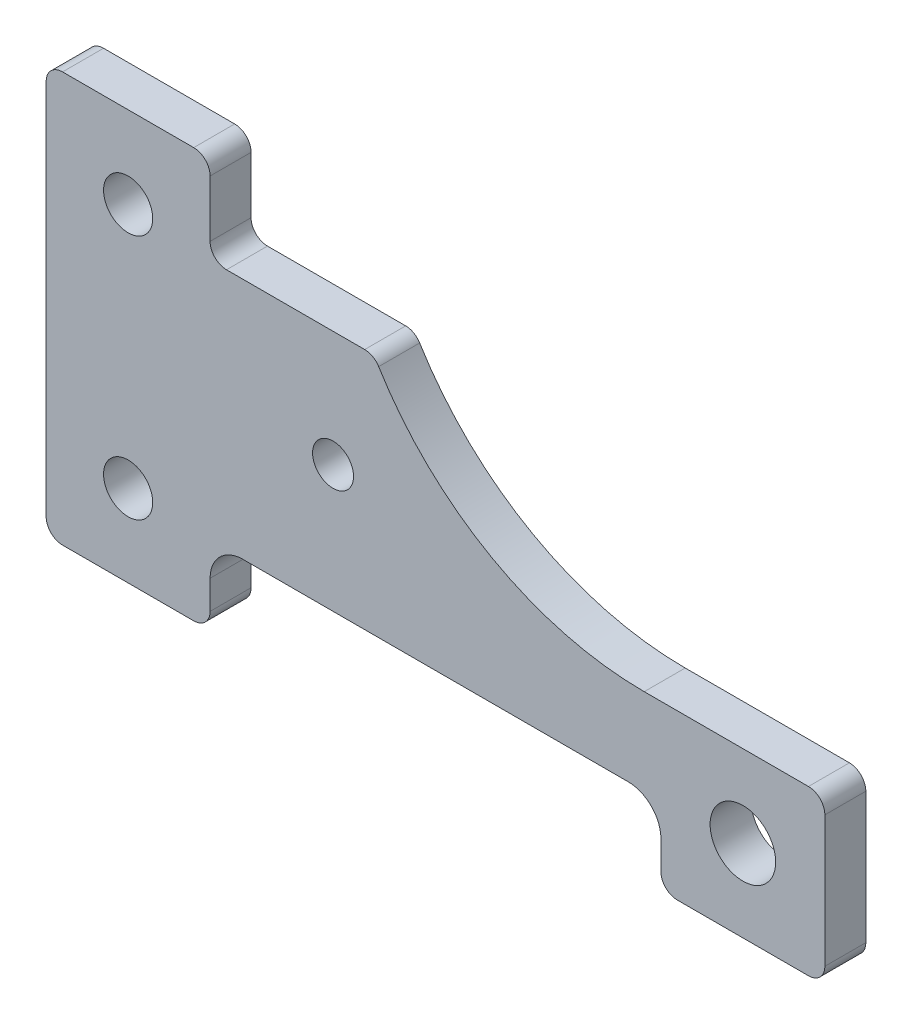
SolidWorks part; units mm, degrees
material "Plain Carbon Steel"
ref_plane "Front Plane" through (0, 0, 0) normal (0, 0, 1) x (1, 0, 0)
ref_plane "Top Plane" through (0, 0, 0) normal (0, 1, 0) x (1, 0, 0)
ref_plane "Right Plane" through (0, 0, 0) normal (1, 0, 0) x (0, 0, -1)
sketch "Bracket Profile Sketch" plane through (0, 0, 0) normal (0, 0, 1) x (1, 0, 0)
  line L0 (-393.3374, 211.3084) -> (-393.3374, -248.6916)
  line L1 (-373.3374, -268.6916) -> (-213.3374, -268.6916)
  line L2 (-193.3374, -248.6916) -> (-193.3374, -213.676)
  line L3 (-153.3374, -173.676) -> (316.6626, -173.676)
  line L4 (356.6626, -213.676) -> (356.6626, -248.6916)
  line L5 (376.6626, -268.6916) -> (536.6626, -268.6916)
  line L6 (556.6626, -248.6916) -> (556.6626, -88.6916)
  line L7 (536.6626, -68.6916) -> (336.308, -68.6916)
  line L8 (-193.3374, 211.3084) -> (-193.3374, 142.2741)
  line L9 (-173.3374, 122.2741) -> (-4.7267, 122.2741)
  line L10 (-373.3374, 231.3084) -> (-213.3374, 231.3084)
  arc A0 (336.308, -68.6916) -> (12.325, 112.7259) centre (336.308, 311.3084) cw
  arc A1 (316.6626, -173.676) -> (356.6626, -213.676) centre (316.6626, -213.676) cw
  arc A2 (-193.3374, -213.676) -> (-153.3374, -173.676) centre (-153.3374, -213.676) cw
  arc A3 (-213.3374, -268.6916) -> (-193.3374, -248.6916) centre (-213.3374, -248.6916) ccw
  arc A4 (356.6626, -248.6916) -> (376.6626, -268.6916) centre (376.6626, -248.6916) ccw
  arc A5 (536.6626, -268.6916) -> (556.6626, -248.6916) centre (536.6626, -248.6916) ccw
  arc A6 (556.6626, -88.6916) -> (536.6626, -68.6916) centre (536.6626, -88.6916) ccw
  arc A7 (-4.7267, 122.2741) -> (12.325, 112.7259) centre (-4.7267, 102.2741) cw
  arc A8 (-193.3374, 142.2741) -> (-173.3374, 122.2741) centre (-173.3374, 142.2741) ccw
  arc A9 (-193.3374, 211.3084) -> (-213.3374, 231.3084) centre (-213.3374, 211.3084) ccw
  arc A10 (-393.3374, 211.3084) -> (-373.3374, 231.3084) centre (-373.3374, 211.3084) cw
  arc A11 (-393.3374, -248.6916) -> (-373.3374, -268.6916) centre (-373.3374, -248.6916) ccw
  circle A12 centre (-293.3374, 131.3084) radius 30
  circle A13 centre (-293.3374, -168.6916) radius 30
  circle A14 centre (-43.3374, -18.6916) radius 25
  circle A15 centre (456.6626, -168.6916) radius 40
  point P18 (-193.3374, -173.676)
  point P21 (-193.3374, -268.6916)
  point P24 (356.6626, -268.6916)
  point P27 (556.6626, -268.6916)
  point P30 (556.6626, -68.6916)
  point P33 (6.6626, 122.2741)
  point P36 (-193.3374, 122.2741)
  point P39 (-193.3374, 231.3084)
  point P42 (-393.3374, 231.3084)
  point P45 (-393.3374, -268.6916)
  dimension "D7" = 380
  dimension "D8" = 40
  dimension "D9" = 20
  dimension "D11" = 50
  dimension "D12" = 60
  dimension "D13" = 150
  dimension "60" = 60
  dimension "D16" = 80
  dimension "D1" = 500
  dimension "D2" = 200
  dimension "D3" = 200
  dimension "D4" = 200
  dimension "D5" = 200
  dimension "D6" = 200
  dimension "950" = 950
  dimension "D10" = 100
  dimension "100" = 100
  dimension "D14" = 100
  dimension "D15" = 100
  dimension "D17" = 95.0156
  dimension "D18" = 109.0343
  dimension "D19" = 100
  dimension "D20" = 250
  dimension "D21" = 393.3374
  dimension "D22" = 268.6916
extrude "Bracket Plate 50mm" add sketch "Bracket Profile Sketch" along normal mid plane 50
